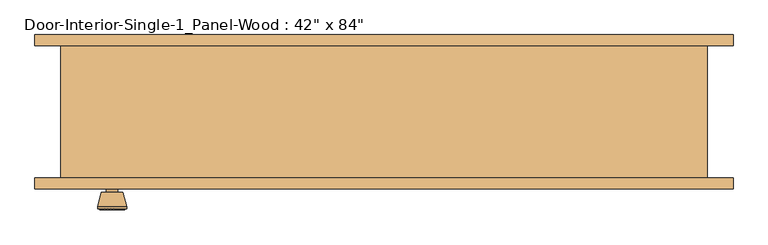
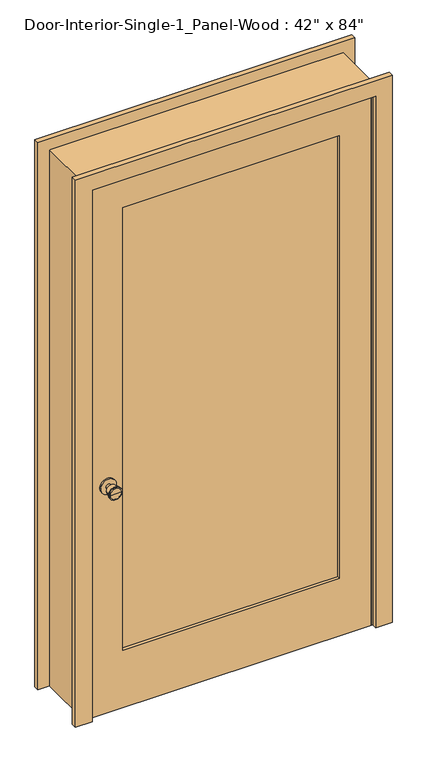
"""IFC4 building model written with IfcOpenShell, lengths in millimetres: door geometry."""

from ifc_helpers import new_model, si_unit, point, frame, frame_2d, origin, place, context, project, spatial, polyline, circle_curve, trimmed, segment, composite_curve, outline, extrude, faceted_brep, source, transform, mapped, element, save
from ifc_brep_helpers import plane_surface, cylinder_surface, revolved_surface, advanced_brep


def door_0f538abb(model_context):
    return source(origin(), model_context, "Body", "SolidModel", [
        advanced_brep(
        [(-469.9, -70.2, 914.4), (-479.9, -70.2, 914.4), (-459.9, -70.2, 914.4), (-449.4241324, -21.2, 914.4), (-490.3758676, -21.2, 914.4), (-469.9, -21.2, 914.4), (-444.9, -23.0278681, 914.4), (-494.9, -23.0278681, 914.4), (-444.9, -26.4915463, 914.4), (-494.9, -26.4915463, 914.4), (-451.263764, -51.2, 914.4), (-488.536236, -51.2, 914.4), (-459.9, -51.2, 914.4), (-479.9, -51.2, 914.4)],
        [
            (0, 1),
            (1, 2, circle_curve(frame((-469.9, -70.2, 914.4), z_axis=(0.0, -1.0, 0.0), x_axis=(-1.0, 0.0, 0.0)), 10.0)),
            (2, 0),
            (2, 1, circle_curve(frame((-469.9, -70.2, 914.4), z_axis=(0.0, -1.0, 0.0), x_axis=(-1.0, 0.0, 0.0)), 10.0)),
            (3, 4, circle_curve(frame((-469.9, -21.2, 914.4), z_axis=(0.0, 1.0, 0.0), x_axis=(-1.0, 0.0, 0.0)), 20.4758676)),
            (4, 5),
            (5, 3),
            (4, 3, circle_curve(frame((-469.9, -21.2, 914.4), z_axis=(0.0, 1.0, 0.0), x_axis=(-1.0, 0.0, 0.0)), 20.4758676)),
            (6, 7, circle_curve(frame((-469.9, -23.0278681, 914.4), z_axis=(0.0, 1.0, 0.0), x_axis=(-1.0, 0.0, 0.0)), 25.0)),
            (7, 4),
            (3, 6),
            (7, 6, circle_curve(frame((-469.9, -23.0278681, 914.4), z_axis=(0.0, 1.0, 0.0), x_axis=(-1.0, 0.0, 0.0)), 25.0)),
            (8, 9, circle_curve(frame((-469.9, -26.4915463, 914.4), z_axis=(0.0, 1.0, 0.0), x_axis=(-1.0, 0.0, 0.0)), 25.0)),
            (9, 7),
            (6, 8),
            (9, 8, circle_curve(frame((-469.9, -26.4915463, 914.4), z_axis=(0.0, 1.0, 0.0), x_axis=(-1.0, 0.0, 0.0)), 25.0)),
            (10, 11, circle_curve(frame((-469.9, -51.2, 914.4), z_axis=(0.0, 1.0, 0.0), x_axis=(-1.0, 0.0, 0.0)), 18.636236)),
            (11, 9),
            (8, 10),
            (11, 10, circle_curve(frame((-469.9, -51.2, 914.4), z_axis=(0.0, 1.0, 0.0), x_axis=(-1.0, 0.0, 0.0)), 18.636236)),
            (12, 13, circle_curve(frame((-469.9, -51.2, 914.4), z_axis=(0.0, 1.0, 0.0), x_axis=(-1.0, 0.0, 0.0)), 10.0)),
            (13, 11),
            (10, 12),
            (13, 12, circle_curve(frame((-469.9, -51.2, 914.4), z_axis=(0.0, 1.0, 0.0), x_axis=(-1.0, 0.0, 0.0)), 10.0)),
            (1, 13),
            (12, 2),
        ],
        [
            plane_surface(frame((-469.9, -70.2, 914.4), z_axis=(0.0, -1.0, 0.0), x_axis=(-1.0, 0.0, 0.0))),
            plane_surface(frame((-469.9, -21.2, 914.4), z_axis=(0.0, 1.0, 0.0), x_axis=(-1.0, 0.0, 0.0))),
            revolved_surface(polyline([(-490.3758676, -21.2, 914.4), (-494.9, -23.0278681, 914.4)]), (-469.9, -70.2, 914.4), (0.0, -1.0, 0.0)),
            cylinder_surface(frame((-469.9, -70.2, 914.4), z_axis=(0.0, -1.0, 0.0), x_axis=(-1.0, 0.0, 0.0)), 25.0),
            revolved_surface(polyline([(-494.9, -26.4915463, 914.4), (-488.536236, -51.2, 914.4)]), (-469.9, -70.2, 914.4), (0.0, -1.0, 0.0)),
            plane_surface(frame((-469.9, -51.2, 914.4), z_axis=(0.0, -1.0, 0.0), x_axis=(-1.0, 0.0, 0.0))),
            cylinder_surface(frame((-469.9, -70.2, 914.4), z_axis=(0.0, -1.0, 0.0), x_axis=(-1.0, 0.0, 0.0)), 10.0),
        ],
        [
            (0, [[1, 2, 3]]),
            (0, [[-3, 4, -1]]),
            (1, [[5, 6, 7]]),
            (1, [[8, -7, -6]]),
            (2, [[9, 10, -5, 11]]),
            (2, [[12, -11, -8, -10]]),
            (3, [[13, 14, -9, 15]]),
            (3, [[16, -15, -12, -14]]),
            (4, [[17, 18, -13, 19]]),
            (4, [[20, -19, -16, -18]]),
            (5, [[21, 22, -17, 23]]),
            (5, [[24, -23, -20, -22]]),
            (6, [[-2, 25, -21, 26]]),
            (6, [[-4, -26, -24, -25]]),
        ],
    ),
        extrude(outline(composite_curve([segment(trimmed(circle_curve(frame_2d((914.4, -469.9)), 30.0), [point((914.4, -499.9))], [point((914.4, -439.9))], False, "CARTESIAN"), True, "CONTINUOUS"), segment(trimmed(circle_curve(frame_2d((914.4, -469.9)), 30.0), [point((914.4, -439.9))], [point((914.4, -499.9))], False, "CARTESIAN"), True, "CONTINUOUS")], self_intersect=False)), frame((0.0, -76.2, 0.0), z_axis=(0.0, 1.0, 0.0), x_axis=(0.0, 0.0, 1.0)), (0.0, 0.0, 1.0), 6.0),
        advanced_brep(
        [(-469.9, -117.125, 914.4), (-459.9, -117.125, 914.4), (-479.9, -117.125, 914.4), (-449.4241324, -166.125, 914.4), (-469.9, -166.125, 914.4), (-490.3758676, -166.125, 914.4), (-444.9, -164.2971319, 914.4), (-494.9, -164.2971319, 914.4), (-444.9, -160.8334537, 914.4), (-494.9, -160.8334537, 914.4), (-451.263764, -136.125, 914.4), (-488.536236, -136.125, 914.4), (-459.9, -136.125, 914.4), (-479.9, -136.125, 914.4)],
        [
            (0, 1),
            (1, 2, circle_curve(frame((-469.9, -117.125, 914.4), z_axis=(0.0, 1.0, 0.0), x_axis=(-1.0, 0.0, 0.0)), 10.0)),
            (2, 0),
            (2, 1, circle_curve(frame((-469.9, -117.125, 914.4), z_axis=(0.0, 1.0, 0.0), x_axis=(-1.0, 0.0, 0.0)), 10.0)),
            (3, 4),
            (4, 5),
            (5, 3, circle_curve(frame((-469.9, -166.125, 914.4), z_axis=(0.0, -1.0, 0.0), x_axis=(-1.0, 0.0, 0.0)), 20.4758676)),
            (3, 5, circle_curve(frame((-469.9, -166.125, 914.4), z_axis=(0.0, -1.0, 0.0), x_axis=(-1.0, 0.0, 0.0)), 20.4758676)),
            (6, 3),
            (5, 7),
            (7, 6, circle_curve(frame((-469.9, -164.2971319, 914.4), z_axis=(0.0, -1.0, 0.0), x_axis=(-1.0, 0.0, 0.0)), 25.0)),
            (6, 7, circle_curve(frame((-469.9, -164.2971319, 914.4), z_axis=(0.0, -1.0, 0.0), x_axis=(-1.0, 0.0, 0.0)), 25.0)),
            (8, 6),
            (7, 9),
            (9, 8, circle_curve(frame((-469.9, -160.8334537, 914.4), z_axis=(0.0, -1.0, 0.0), x_axis=(-1.0, 0.0, 0.0)), 25.0)),
            (8, 9, circle_curve(frame((-469.9, -160.8334537, 914.4), z_axis=(0.0, -1.0, 0.0), x_axis=(-1.0, 0.0, 0.0)), 25.0)),
            (10, 8),
            (9, 11),
            (11, 10, circle_curve(frame((-469.9, -136.125, 914.4), z_axis=(0.0, -1.0, 0.0), x_axis=(-1.0, 0.0, 0.0)), 18.636236)),
            (10, 11, circle_curve(frame((-469.9, -136.125, 914.4), z_axis=(0.0, -1.0, 0.0), x_axis=(-1.0, 0.0, 0.0)), 18.636236)),
            (12, 10),
            (11, 13),
            (13, 12, circle_curve(frame((-469.9, -136.125, 914.4), z_axis=(0.0, -1.0, 0.0), x_axis=(-1.0, 0.0, 0.0)), 10.0)),
            (12, 13, circle_curve(frame((-469.9, -136.125, 914.4), z_axis=(0.0, -1.0, 0.0), x_axis=(-1.0, 0.0, 0.0)), 10.0)),
            (1, 12),
            (13, 2),
        ],
        [
            plane_surface(frame((-469.9, -117.125, 914.4), z_axis=(0.0, 1.0, 0.0), x_axis=(-1.0, 0.0, 0.0))),
            plane_surface(frame((-469.9, -166.125, 914.4), z_axis=(0.0, -1.0, 0.0), x_axis=(-1.0, 0.0, 0.0))),
            revolved_surface(polyline([(-490.3758676, -166.125, 914.4), (-494.9, -164.2971319, 914.4)]), (-469.9, -117.125, 914.4), (0.0, 1.0, 0.0)),
            cylinder_surface(frame((-469.9, -117.125, 914.4), z_axis=(0.0, 1.0, 0.0), x_axis=(-1.0, 0.0, 0.0)), 25.0),
            revolved_surface(polyline([(-494.9, -160.8334537, 914.4), (-488.536236, -136.125, 914.4)]), (-469.9, -117.125, 914.4), (0.0, 1.0, 0.0)),
            plane_surface(frame((-469.9, -136.125, 914.4), z_axis=(0.0, 1.0, 0.0), x_axis=(-1.0, 0.0, 0.0))),
            cylinder_surface(frame((-469.9, -117.125, 914.4), z_axis=(0.0, 1.0, 0.0), x_axis=(-1.0, 0.0, 0.0)), 10.0),
        ],
        [
            (0, [[1, 2, 3]]),
            (0, [[-3, 4, -1]]),
            (1, [[5, 6, 7]]),
            (1, [[-6, -5, 8]]),
            (2, [[9, -7, 10, 11]]),
            (2, [[-10, -8, -9, 12]]),
            (3, [[13, -11, 14, 15]]),
            (3, [[-14, -12, -13, 16]]),
            (4, [[17, -15, 18, 19]]),
            (4, [[-18, -16, -17, 20]]),
            (5, [[21, -19, 22, 23]]),
            (5, [[-22, -20, -21, 24]]),
            (6, [[25, -23, 26, -2]]),
            (6, [[-26, -24, -25, -4]]),
        ],
    ),
        extrude(outline(composite_curve([segment(trimmed(circle_curve(frame_2d((914.4, -469.9)), 30.0), [point((914.4, -499.9))], [point((914.4, -439.9))], False, "CARTESIAN"), True, "CONTINUOUS"), segment(trimmed(circle_curve(frame_2d((914.4, -469.9)), 30.0), [point((914.4, -439.9))], [point((914.4, -499.9))], False, "CARTESIAN"), True, "CONTINUOUS")], self_intersect=False)), frame((0.0, -117.125, 0.0), z_axis=(0.0, 1.0, 0.0), x_axis=(0.0, 0.0, 1.0)), (0.0, 0.0, 1.0), 6.0),
        faceted_brep([(558.8, -111.125, 0.0), (533.4, -111.125, 0.0), (533.4, -76.2, 0.0), (520.7, -76.2, 0.0), (520.7, -41.275, 0.0), (533.4, -41.275, 0.0), (533.4, 117.475, 0.0), (558.8, 117.475, 0.0), (558.8, 117.475, 2159.0), (558.8, -111.125, 2159.0), (533.4, 117.475, 2133.6), (-533.4, 117.475, 2133.6), (-533.4, 117.475, 0.0), (-558.8, 117.475, 0.0), (-558.8, 117.475, 2159.0), (533.4, -41.275, 2133.6), (520.7, -41.275, 2120.9), (-520.7, -41.275, 2120.9), (-520.7, -41.275, 0.0), (-533.4, -41.275, 0.0), (-533.4, -41.275, 2133.6), (520.7, -76.2, 2120.9), (533.4, -76.2, 2133.6), (-533.4, -76.2, 2133.6), (-533.4, -76.2, 0.0), (-520.7, -76.2, 0.0), (-520.7, -76.2, 2120.9), (533.4, -111.125, 2133.6), (-558.8, -111.125, 2159.0), (-558.8, -111.125, 0.0), (-533.4, -111.125, 0.0), (-533.4, -111.125, 2133.6)], [[[0, 1, 2, 3, 4, 5, 6, 7]], [[7, 8, 9, 0]], [[6, 10, 11, 12, 13, 14, 8, 7]], [[5, 15, 10, 6]], [[4, 16, 17, 18, 19, 20, 15, 5]], [[3, 21, 16, 4]], [[2, 22, 23, 24, 25, 26, 21, 3]], [[1, 27, 22, 2]], [[0, 9, 28, 29, 30, 31, 27, 1]], [[8, 14, 28, 9]], [[15, 20, 11, 10]], [[21, 26, 17, 16]], [[27, 31, 23, 22]], [[29, 13, 12, 19, 18, 25, 24, 30]], [[14, 13, 29, 28]], [[20, 19, 12, 11]], [[26, 25, 18, 17]], [[31, 30, 24, 23]]]),
        extrude(outline(polyline([(2133.6, -533.4), (0.0, -533.4), (0.0, 533.4), (2133.6, 533.4), (2133.6, -533.4)]), holes=[polyline([(2014.5375, -412.75), (2014.5375, 412.75), (231.775, 412.75), (231.775, -412.75), (2014.5375, -412.75)])]), frame((0.0, -111.125, 0.0), z_axis=(0.0, 1.0, 0.0), x_axis=(0.0, 0.0, 1.0)), (0.0, 0.0, 1.0), 34.925),
        extrude(outline(polyline([(412.75, -87.8416667), (412.75, -99.4833333), (-412.75, -99.4833333), (-412.75, -87.8416667), (412.75, -87.8416667)])), frame((0.0, 0.0, 231.775), z_axis=(0.0, 0.0, 1.0), x_axis=(1.0, 0.0, 0.0)), (0.0, 0.0, 1.0), 1782.7625),
        extrude(outline(polyline([(0.0, 603.25), (2203.45, 603.25), (2203.45, -603.25), (0.0, -603.25), (0.0, -539.75), (2139.95, -539.75), (2139.95, 539.75), (0.0, 539.75), (0.0, 603.25)])), frame((0.0, -130.175, 0.0), z_axis=(0.0, 1.0, 0.0), x_axis=(0.0, 0.0, 1.0)), (0.0, 0.0, 1.0), 19.05),
        extrude(outline(polyline([(0.0, 603.25), (2203.45, 603.25), (2203.45, -603.25), (0.0, -603.25), (0.0, -539.75), (2139.95, -539.75), (2139.95, 539.75), (0.0, 539.75), (0.0, 603.25)])), frame((0.0, 117.475, 0.0), z_axis=(0.0, 1.0, 0.0), x_axis=(0.0, 0.0, 1.0)), (0.0, 0.0, 1.0), 19.05),
    ])


if __name__ == "__main__":
    model = new_model("IFC4")
    model_context = context("Model", 3, world=origin())
    ifc_project = project(units=[si_unit("LENGTHUNIT", "METRE", prefix="MILLI")], contexts=[model_context])
    site = spatial("IfcSite", under=ifc_project)
    building = spatial("IfcBuilding", under=site)
    placement = place(None, origin())
    door_shape = door_0f538abb(model_context)
    element("IfcDoor", 1, ObjectType="Door-Interior-Single-1_Panel-Wood : 42\" x 84\"", at=placement, inside=building, context=model_context, shape_type="MappedRepresentation", body=[
        mapped(door_shape, transform((0.0, 0.0, 0.0), x_axis=(1.0, 0.0, 0.0), y_axis=(0.0, 1.0, 0.0), z_axis=(0.0, 0.0, 1.0))),
    ])
    save(model, "model.ifc")

# Revit data of these elements
# Type "Door-Interior-Single-1_Panel-Wood : 42\" x 84\""
#   Type Mark = "9"
#   Assembly Code = "C1020300"
#   Analytic Construction = "Wooden"
#   Top Rail = 0' - 4 11/16"
#   Thickness = 0' - 1 3/8"
#   Thermal Resistance (R) = 2.5876 (h·ft²·°F)/BTU
#   Swing Angle [instance default] = 90.00°
#   Stiles = 0' - 4 3/4"
#   Rough Width = 3' - 8"
#   Rough Height = 7' - 1"
#   Height = 7' - 0"
#   Width = 3' - 6"
#   Heat Transfer Coefficient (U) = 0.3865 BTU/(h·ft²·°F)
#   Bottom Rail = 0' - 9 1/8"
#   Trim Material = Cherry
#   Panel Material = Cherry
#   Frame Material = Cherry
#   Door Handle Material = Aluminum
#   Visual Light Transmittance = 0
#   Solar Heat Gain Coefficient = 0
#   Wall Closure = (empty or 0)
#   Function = (empty or 0)
# Element 1 (IfcDoor, "Door-Interior-Single-1_Panel-Wood : 42\" x 84\"")
#   Materials on its faces: "Cherry", "Aluminum"
# Materials
#   "Cherry": class "Wood", colour RGB 226 177 128, transparency 0, Description = "Prunus Serotina", Cost = 0
#   "Aluminum": class "Metal", colour RGB 247 247 247, transparency 0, Description = "Aluminum 6061", Cost = 0
